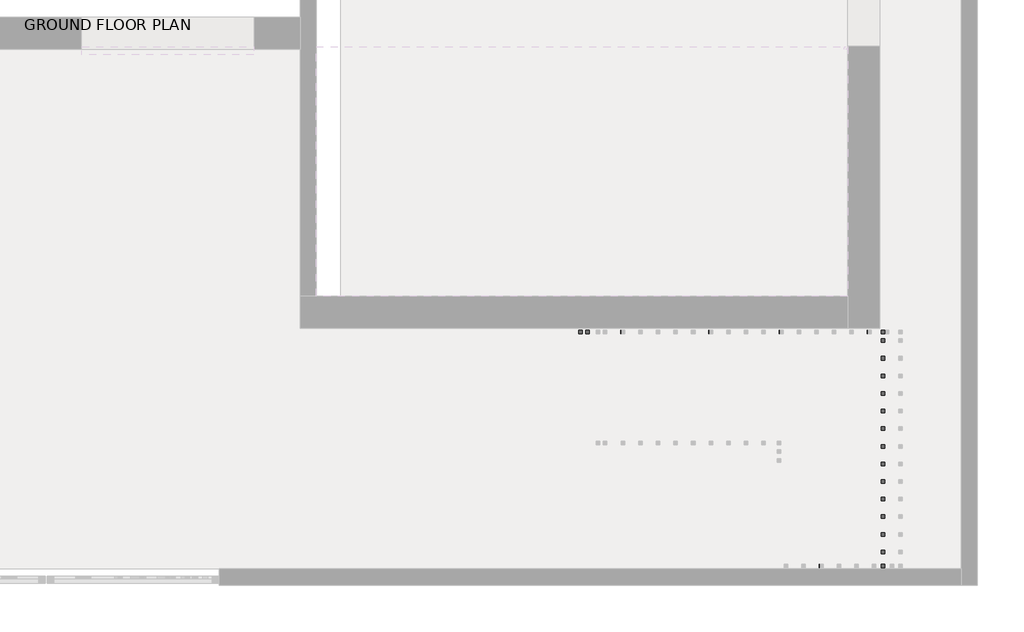
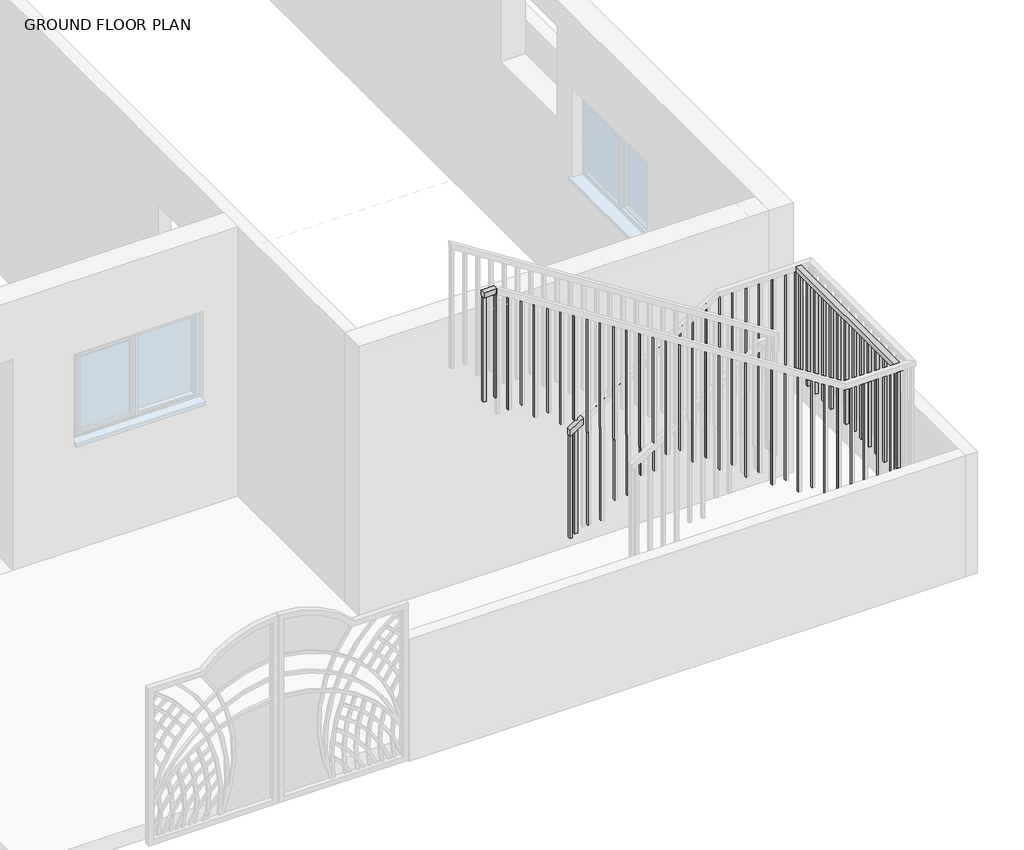
# One storey, part 6 of 23: 2 railings.
"""IFC4 building model written with IfcOpenShell, lengths in millimetres."""

from ifc_helpers import new_model, si_unit, frame, origin, place, context, project, spatial, polyline, outline, extrude, faceted_brep, element, save

model = new_model("IFC4")

# Units and contexts
model_context = context("Model", 3, world=origin())
ifc_project = project(units=[si_unit("LENGTHUNIT", "METRE", prefix="MILLI")], contexts=[model_context])

# Site, building, storey
site = spatial("IfcSite", under=ifc_project)
building = spatial("IfcBuilding", under=site)
storey = spatial("IfcBuildingStorey", under=building, Name="GROUND FLOOR PLAN", Elevation=487.68)

# Railings
placement = place(None, origin())
element("IfcRailing", 1, ObjectType="1100mm", at=placement, inside=storey, context=model_context, shape_type="SolidModel", body=[
    faceted_brep([(-8805.870786, -10220.0521308, 1832.3649576), (-8805.870786, -10220.0521308, 1773.007357), (-8805.870786, -10270.0521308, 1773.007357), (-8805.870786, -10270.0521308, 1832.3649576), (-7409.7306254, -10220.0521308, 2725.6), (-7395.1045513, -10220.0521308, 2675.6), (-7395.1045513, -10270.0521308, 2675.6), (-7409.7306254, -10270.0521308, 2725.6), (-6621.5344696, -10220.0521308, 2725.6), (-6621.5344696, -10220.0521308, 2675.6), (-6671.5344696, -10270.0521308, 2675.6), (-6671.5344696, -10270.0521308, 2725.6), (-6621.5344696, -11933.6860066, 2725.6), (-6621.5344696, -11933.6860066, 2675.6), (-6671.5344696, -11883.6860066, 2675.6), (-6671.5344696, -11883.6860066, 2725.6), (-7155.718398, -11933.6860066, 2725.6), (-7170.3479429, -11933.6860066, 2675.6), (-7170.3479429, -11883.6860066, 2675.6), (-7155.718398, -11883.6860066, 2725.6), (-10457.8773536, -11933.6860066, 4838.88), (-10472.5068984, -11933.6860066, 4788.88), (-10472.5068984, -11883.6860066, 4788.88), (-10457.8773536, -11883.6860066, 4838.88), (-10583.5985666, -11933.6860066, 4838.88), (-10583.5985666, -11883.6860066, 4838.88), (-10583.5985666, -11883.6860066, 4788.88), (-10583.5985666, -11933.6860066, 4788.88)], [[[0, 1, 2, 3]], [[1, 0, 4, 5]], [[2, 1, 5, 6]], [[3, 2, 6, 7]], [[0, 3, 7, 4]], [[5, 4, 8, 9]], [[6, 5, 9, 10]], [[7, 6, 10, 11]], [[4, 7, 11, 8]], [[9, 8, 12, 13]], [[10, 9, 13, 14]], [[11, 10, 14, 15]], [[8, 11, 15, 12]], [[13, 12, 16, 17]], [[14, 13, 17, 18]], [[15, 14, 18, 19]], [[12, 15, 19, 16]], [[17, 16, 20, 21]], [[18, 17, 21, 22]], [[19, 18, 22, 23]], [[16, 19, 23, 20]], [[24, 25, 26, 27]], [[21, 20, 24, 27]], [[22, 21, 27, 26]], [[23, 22, 26, 25]], [[20, 23, 25, 24]]]),
    extrude(outline(polyline([(-10446.5344696, -11921.1860066), (-10471.5344696, -11921.1860066), (-10471.5344696, -11896.1860066), (-10446.5344696, -11896.1860066), (-10446.5344696, -11921.1860066)])), frame((0.0, 0.0, 3738.88), z_axis=(0.0, 0.0, 1.0), x_axis=(1.0, 0.0, 0.0)), (0.0, 0.0, 1.0), 1050.0),
    extrude(outline(polyline([(4692.2622966, -10321.5344696), (4708.2615264, -10346.5344696), (3576.32, -10346.5344696), (3576.32, -10321.5344696), (4692.2622966, -10321.5344696)])), frame((0.0, -11921.1860066, 0.0), z_axis=(0.0, 1.0, 0.0), x_axis=(0.0, 0.0, 1.0)), (0.0, 0.0, 1.0), 25.0),
    extrude(outline(polyline([(4612.2661476, -10196.5344696), (4628.2653774, -10221.5344696), (3576.32, -10221.5344696), (3576.32, -10196.5344696), (4612.2661476, -10196.5344696)])), frame((0.0, -11921.1860066, 0.0), z_axis=(0.0, 1.0, 0.0), x_axis=(0.0, 0.0, 1.0)), (0.0, 0.0, 1.0), 25.0),
    extrude(outline(polyline([(4532.2699985, -10071.5344696), (4548.2692283, -10096.5344696), (3413.76, -10096.5344696), (3413.76, -10071.5344696), (4532.2699985, -10071.5344696)])), frame((0.0, -11921.1860066, 0.0), z_axis=(0.0, 1.0, 0.0), x_axis=(0.0, 0.0, 1.0)), (0.0, 0.0, 1.0), 25.0),
    extrude(outline(polyline([(4452.2738495, -9946.5344696), (4468.2730793, -9971.5344696), (3413.76, -9971.5344696), (3413.76, -9946.5344696), (4452.2738495, -9946.5344696)])), frame((0.0, -11921.1860066, 0.0), z_axis=(0.0, 1.0, 0.0), x_axis=(0.0, 0.0, 1.0)), (0.0, 0.0, 1.0), 25.0),
    extrude(outline(polyline([(4372.2777004, -9821.5344696), (4388.2769302, -9846.5344696), (3251.2, -9846.5344696), (3251.2, -9821.5344696), (4372.2777004, -9821.5344696)])), frame((0.0, -11921.1860066, 0.0), z_axis=(0.0, 1.0, 0.0), x_axis=(0.0, 0.0, 1.0)), (0.0, 0.0, 1.0), 25.0),
    extrude(outline(polyline([(4292.2815514, -9696.5344696), (4308.2807812, -9721.5344696), (3251.2, -9721.5344696), (3251.2, -9696.5344696), (4292.2815514, -9696.5344696)])), frame((0.0, -11921.1860066, 0.0), z_axis=(0.0, 1.0, 0.0), x_axis=(0.0, 0.0, 1.0)), (0.0, 0.0, 1.0), 25.0),
    extrude(outline(polyline([(4212.2854023, -9571.5344696), (4228.2846321, -9596.5344696), (3088.64, -9596.5344696), (3088.64, -9571.5344696), (4212.2854023, -9571.5344696)])), frame((0.0, -11921.1860066, 0.0), z_axis=(0.0, 1.0, 0.0), x_axis=(0.0, 0.0, 1.0)), (0.0, 0.0, 1.0), 25.0),
    extrude(outline(polyline([(4132.2892533, -9446.5344696), (4148.2884831, -9471.5344696), (3088.64, -9471.5344696), (3088.64, -9446.5344696), (4132.2892533, -9446.5344696)])), frame((0.0, -11921.1860066, 0.0), z_axis=(0.0, 1.0, 0.0), x_axis=(0.0, 0.0, 1.0)), (0.0, 0.0, 1.0), 25.0),
    extrude(outline(polyline([(4052.2931042, -9321.5344696), (4068.292334, -9346.5344696), (2926.08, -9346.5344696), (2926.08, -9321.5344696), (4052.2931042, -9321.5344696)])), frame((0.0, -11921.1860066, 0.0), z_axis=(0.0, 1.0, 0.0), x_axis=(0.0, 0.0, 1.0)), (0.0, 0.0, 1.0), 25.0),
    extrude(outline(polyline([(3972.2969552, -9196.5344696), (3988.296185, -9221.5344696), (2926.08, -9221.5344696), (2926.08, -9196.5344696), (3972.2969552, -9196.5344696)])), frame((0.0, -11921.1860066, 0.0), z_axis=(0.0, 1.0, 0.0), x_axis=(0.0, 0.0, 1.0)), (0.0, 0.0, 1.0), 25.0),
    extrude(outline(polyline([(3892.3008061, -9071.5344696), (3908.3000359, -9096.5344696), (2763.52, -9096.5344696), (2763.52, -9071.5344696), (3892.3008061, -9071.5344696)])), frame((0.0, -11921.1860066, 0.0), z_axis=(0.0, 1.0, 0.0), x_axis=(0.0, 0.0, 1.0)), (0.0, 0.0, 1.0), 25.0),
    extrude(outline(polyline([(3812.3046571, -8946.5344696), (3828.3038869, -8971.5344696), (2763.52, -8971.5344696), (2763.52, -8946.5344696), (3812.3046571, -8946.5344696)])), frame((0.0, -11921.1860066, 0.0), z_axis=(0.0, 1.0, 0.0), x_axis=(0.0, 0.0, 1.0)), (0.0, 0.0, 1.0), 25.0),
    extrude(outline(polyline([(3732.308508, -8821.5344696), (3748.3077378, -8846.5344696), (2600.96, -8846.5344696), (2600.96, -8821.5344696), (3732.308508, -8821.5344696)])), frame((0.0, -11921.1860066, 0.0), z_axis=(0.0, 1.0, 0.0), x_axis=(0.0, 0.0, 1.0)), (0.0, 0.0, 1.0), 25.0),
    extrude(outline(polyline([(3652.312359, -8696.5344696), (3668.3115888, -8721.5344696), (2600.96, -8721.5344696), (2600.96, -8696.5344696), (3652.312359, -8696.5344696)])), frame((0.0, -11921.1860066, 0.0), z_axis=(0.0, 1.0, 0.0), x_axis=(0.0, 0.0, 1.0)), (0.0, 0.0, 1.0), 25.0),
    extrude(outline(polyline([(3572.3162099, -8571.5344696), (3588.3154397, -8596.5344696), (2438.4, -8596.5344696), (2438.4, -8571.5344696), (3572.3162099, -8571.5344696)])), frame((0.0, -11921.1860066, 0.0), z_axis=(0.0, 1.0, 0.0), x_axis=(0.0, 0.0, 1.0)), (0.0, 0.0, 1.0), 25.0),
    extrude(outline(polyline([(3492.3200609, -8446.5344696), (3508.3192907, -8471.5344696), (2438.4, -8471.5344696), (2438.4, -8446.5344696), (3492.3200609, -8446.5344696)])), frame((0.0, -11921.1860066, 0.0), z_axis=(0.0, 1.0, 0.0), x_axis=(0.0, 0.0, 1.0)), (0.0, 0.0, 1.0), 25.0),
    extrude(outline(polyline([(3412.3239118, -8321.5344696), (3428.3231416, -8346.5344696), (2275.84, -8346.5344696), (2275.84, -8321.5344696), (3412.3239118, -8321.5344696)])), frame((0.0, -11921.1860066, 0.0), z_axis=(0.0, 1.0, 0.0), x_axis=(0.0, 0.0, 1.0)), (0.0, 0.0, 1.0), 25.0),
    extrude(outline(polyline([(3332.3277628, -8196.5344696), (3348.3269926, -8221.5344696), (2275.84, -8221.5344696), (2275.84, -8196.5344696), (3332.3277628, -8196.5344696)])), frame((0.0, -11921.1860066, 0.0), z_axis=(0.0, 1.0, 0.0), x_axis=(0.0, 0.0, 1.0)), (0.0, 0.0, 1.0), 25.0),
    extrude(outline(polyline([(3252.3316137, -8071.5344696), (3268.3308435, -8096.5344696), (2113.28, -8096.5344696), (2113.28, -8071.5344696), (3252.3316137, -8071.5344696)])), frame((0.0, -11921.1860066, 0.0), z_axis=(0.0, 1.0, 0.0), x_axis=(0.0, 0.0, 1.0)), (0.0, 0.0, 1.0), 25.0),
    extrude(outline(polyline([(3172.3354647, -7946.5344696), (3188.3346945, -7971.5344696), (2113.28, -7971.5344696), (2113.28, -7946.5344696), (3172.3354647, -7946.5344696)])), frame((0.0, -11921.1860066, 0.0), z_axis=(0.0, 1.0, 0.0), x_axis=(0.0, 0.0, 1.0)), (0.0, 0.0, 1.0), 25.0),
    extrude(outline(polyline([(3092.4129874, -7821.5344696), (3108.4077111, -7846.5344696), (1950.72, -7846.5344696), (1950.72, -7821.5344696), (3092.4129874, -7821.5344696)])), frame((0.0, -11921.1860066, 0.0), z_axis=(0.0, 1.0, 0.0), x_axis=(0.0, 0.0, 1.0)), (0.0, 0.0, 1.0), 25.0),
    extrude(outline(polyline([(3012.4393691, -7696.5344696), (3028.4340928, -7721.5344696), (1950.72, -7721.5344696), (1950.72, -7696.5344696), (3012.4393691, -7696.5344696)])), frame((0.0, -11921.1860066, 0.0), z_axis=(0.0, 1.0, 0.0), x_axis=(0.0, 0.0, 1.0)), (0.0, 0.0, 1.0), 25.0),
    extrude(outline(polyline([(2932.4657508, -7571.5344696), (2948.4604745, -7596.5344696), (1788.16, -7596.5344696), (1788.16, -7571.5344696), (2932.4657508, -7571.5344696)])), frame((0.0, -11921.1860066, 0.0), z_axis=(0.0, 1.0, 0.0), x_axis=(0.0, 0.0, 1.0)), (0.0, 0.0, 1.0), 25.0),
    extrude(outline(polyline([(2852.4921325, -7446.5344696), (2868.4868562, -7471.5344696), (1788.16, -7471.5344696), (1788.16, -7446.5344696), (2852.4921325, -7446.5344696)])), frame((0.0, -11921.1860066, 0.0), z_axis=(0.0, 1.0, 0.0), x_axis=(0.0, 0.0, 1.0)), (0.0, 0.0, 1.0), 25.0),
    extrude(outline(polyline([(2772.3547194, -7321.5344696), (2788.3539492, -7346.5344696), (1625.6, -7346.5344696), (1625.6, -7321.5344696), (2772.3547194, -7321.5344696)])), frame((0.0, -11921.1860066, 0.0), z_axis=(0.0, 1.0, 0.0), x_axis=(0.0, 0.0, 1.0)), (0.0, 0.0, 1.0), 25.0),
    extrude(outline(polyline([(2692.3585703, -7196.5344696), (2708.3578001, -7221.5344696), (1625.6, -7221.5344696), (1625.6, -7196.5344696), (2692.3585703, -7196.5344696)])), frame((0.0, -11921.1860066, 0.0), z_axis=(0.0, 1.0, 0.0), x_axis=(0.0, 0.0, 1.0)), (0.0, 0.0, 1.0), 25.0),
    extrude(outline(polyline([(-7071.5344696, -11921.1860066), (-7096.5344696, -11921.1860066), (-7096.5344696, -11896.1860066), (-7071.5344696, -11896.1860066), (-7071.5344696, -11921.1860066)])), frame((0.0, 0.0, 1625.6), z_axis=(0.0, 0.0, 1.0), x_axis=(1.0, 0.0, 0.0)), (0.0, 0.0, 1.0), 1050.0),
    extrude(outline(polyline([(-6946.5344696, -11921.1860066), (-6971.5344696, -11921.1860066), (-6971.5344696, -11896.1860066), (-6946.5344696, -11896.1860066), (-6946.5344696, -11921.1860066)])), frame((0.0, 0.0, 1625.6), z_axis=(0.0, 0.0, 1.0), x_axis=(1.0, 0.0, 0.0)), (0.0, 0.0, 1.0), 1050.0),
    extrude(outline(polyline([(-6821.5344696, -11921.1860066), (-6846.5344696, -11921.1860066), (-6846.5344696, -11896.1860066), (-6821.5344696, -11896.1860066), (-6821.5344696, -11921.1860066)])), frame((0.0, 0.0, 1625.6), z_axis=(0.0, 0.0, 1.0), x_axis=(1.0, 0.0, 0.0)), (0.0, 0.0, 1.0), 1050.0),
    extrude(outline(polyline([(-6696.5344696, -11921.1860066), (-6721.5344696, -11921.1860066), (-6721.5344696, -11896.1860066), (-6696.5344696, -11896.1860066), (-6696.5344696, -11921.1860066)])), frame((0.0, 0.0, 1625.6), z_axis=(0.0, 0.0, 1.0), x_axis=(1.0, 0.0, 0.0)), (0.0, 0.0, 1.0), 1050.0),
    extrude(outline(polyline([(-6634.0344696, -11795.0521308), (-6634.0344696, -11820.0521308), (-6659.0344696, -11820.0521308), (-6659.0344696, -11795.0521308), (-6634.0344696, -11795.0521308)])), frame((0.0, 0.0, 1625.6), z_axis=(0.0, 0.0, 1.0), x_axis=(1.0, 0.0, 0.0)), (0.0, 0.0, 1.0), 1050.0),
    extrude(outline(polyline([(-6634.0344696, -11670.0521308), (-6634.0344696, -11695.0521308), (-6659.0344696, -11695.0521308), (-6659.0344696, -11670.0521308), (-6634.0344696, -11670.0521308)])), frame((0.0, 0.0, 1625.6), z_axis=(0.0, 0.0, 1.0), x_axis=(1.0, 0.0, 0.0)), (0.0, 0.0, 1.0), 1050.0),
    extrude(outline(polyline([(-6634.0344696, -11545.0521308), (-6634.0344696, -11570.0521308), (-6659.0344696, -11570.0521308), (-6659.0344696, -11545.0521308), (-6634.0344696, -11545.0521308)])), frame((0.0, 0.0, 1625.6), z_axis=(0.0, 0.0, 1.0), x_axis=(1.0, 0.0, 0.0)), (0.0, 0.0, 1.0), 1050.0),
    extrude(outline(polyline([(-6634.0344696, -11420.0521308), (-6634.0344696, -11445.0521308), (-6659.0344696, -11445.0521308), (-6659.0344696, -11420.0521308), (-6634.0344696, -11420.0521308)])), frame((0.0, 0.0, 1625.6), z_axis=(0.0, 0.0, 1.0), x_axis=(1.0, 0.0, 0.0)), (0.0, 0.0, 1.0), 1050.0),
    extrude(outline(polyline([(-6634.0344696, -11295.0521308), (-6634.0344696, -11320.0521308), (-6659.0344696, -11320.0521308), (-6659.0344696, -11295.0521308), (-6634.0344696, -11295.0521308)])), frame((0.0, 0.0, 1625.6), z_axis=(0.0, 0.0, 1.0), x_axis=(1.0, 0.0, 0.0)), (0.0, 0.0, 1.0), 1050.0),
    extrude(outline(polyline([(-6634.0344696, -11170.0521308), (-6634.0344696, -11195.0521308), (-6659.0344696, -11195.0521308), (-6659.0344696, -11170.0521308), (-6634.0344696, -11170.0521308)])), frame((0.0, 0.0, 1625.6), z_axis=(0.0, 0.0, 1.0), x_axis=(1.0, 0.0, 0.0)), (0.0, 0.0, 1.0), 1050.0),
    extrude(outline(polyline([(-6634.0344696, -11045.0521308), (-6634.0344696, -11070.0521308), (-6659.0344696, -11070.0521308), (-6659.0344696, -11045.0521308), (-6634.0344696, -11045.0521308)])), frame((0.0, 0.0, 1625.6), z_axis=(0.0, 0.0, 1.0), x_axis=(1.0, 0.0, 0.0)), (0.0, 0.0, 1.0), 1050.0),
    extrude(outline(polyline([(-6634.0344696, -10920.0521308), (-6634.0344696, -10945.0521308), (-6659.0344696, -10945.0521308), (-6659.0344696, -10920.0521308), (-6634.0344696, -10920.0521308)])), frame((0.0, 0.0, 1625.6), z_axis=(0.0, 0.0, 1.0), x_axis=(1.0, 0.0, 0.0)), (0.0, 0.0, 1.0), 1050.0),
    extrude(outline(polyline([(-6634.0344696, -10795.0521308), (-6634.0344696, -10820.0521308), (-6659.0344696, -10820.0521308), (-6659.0344696, -10795.0521308), (-6634.0344696, -10795.0521308)])), frame((0.0, 0.0, 1625.6), z_axis=(0.0, 0.0, 1.0), x_axis=(1.0, 0.0, 0.0)), (0.0, 0.0, 1.0), 1050.0),
    extrude(outline(polyline([(-6634.0344696, -10670.0521308), (-6634.0344696, -10695.0521308), (-6659.0344696, -10695.0521308), (-6659.0344696, -10670.0521308), (-6634.0344696, -10670.0521308)])), frame((0.0, 0.0, 1625.6), z_axis=(0.0, 0.0, 1.0), x_axis=(1.0, 0.0, 0.0)), (0.0, 0.0, 1.0), 1050.0),
    extrude(outline(polyline([(-6634.0344696, -10545.0521308), (-6634.0344696, -10570.0521308), (-6659.0344696, -10570.0521308), (-6659.0344696, -10545.0521308), (-6634.0344696, -10545.0521308)])), frame((0.0, 0.0, 1625.6), z_axis=(0.0, 0.0, 1.0), x_axis=(1.0, 0.0, 0.0)), (0.0, 0.0, 1.0), 1050.0),
    extrude(outline(polyline([(-6634.0344696, -10420.0521308), (-6634.0344696, -10445.0521308), (-6659.0344696, -10445.0521308), (-6659.0344696, -10420.0521308), (-6634.0344696, -10420.0521308)])), frame((0.0, 0.0, 1625.6), z_axis=(0.0, 0.0, 1.0), x_axis=(1.0, 0.0, 0.0)), (0.0, 0.0, 1.0), 1050.0),
    extrude(outline(polyline([(-6634.0344696, -10295.0521308), (-6634.0344696, -10320.0521308), (-6659.0344696, -10320.0521308), (-6659.0344696, -10295.0521308), (-6634.0344696, -10295.0521308)])), frame((0.0, 0.0, 1625.6), z_axis=(0.0, 0.0, 1.0), x_axis=(1.0, 0.0, 0.0)), (0.0, 0.0, 1.0), 1050.0),
    extrude(outline(polyline([(-6755.870786, -10232.5521308), (-6730.870786, -10232.5521308), (-6730.870786, -10257.5521308), (-6755.870786, -10257.5521308), (-6755.870786, -10232.5521308)])), frame((0.0, 0.0, 1625.6), z_axis=(0.0, 0.0, 1.0), x_axis=(1.0, 0.0, 0.0)), (0.0, 0.0, 1.0), 1050.0),
    extrude(outline(polyline([(-6880.870786, -10232.5521308), (-6855.870786, -10232.5521308), (-6855.870786, -10257.5521308), (-6880.870786, -10257.5521308), (-6880.870786, -10232.5521308)])), frame((0.0, 0.0, 1625.6), z_axis=(0.0, 0.0, 1.0), x_axis=(1.0, 0.0, 0.0)), (0.0, 0.0, 1.0), 1050.0),
    extrude(outline(polyline([(-7005.870786, -10232.5521308), (-6980.870786, -10232.5521308), (-6980.870786, -10257.5521308), (-7005.870786, -10257.5521308), (-7005.870786, -10232.5521308)])), frame((0.0, 0.0, 1625.6), z_axis=(0.0, 0.0, 1.0), x_axis=(1.0, 0.0, 0.0)), (0.0, 0.0, 1.0), 1050.0),
    extrude(outline(polyline([(-7130.870786, -10232.5521308), (-7105.870786, -10232.5521308), (-7105.870786, -10257.5521308), (-7130.870786, -10257.5521308), (-7130.870786, -10232.5521308)])), frame((0.0, 0.0, 1625.6), z_axis=(0.0, 0.0, 1.0), x_axis=(1.0, 0.0, 0.0)), (0.0, 0.0, 1.0), 1050.0),
    extrude(outline(polyline([(-7255.870786, -10232.5521308), (-7230.870786, -10232.5521308), (-7230.870786, -10257.5521308), (-7255.870786, -10257.5521308), (-7255.870786, -10232.5521308)])), frame((0.0, 0.0, 1625.6), z_axis=(0.0, 0.0, 1.0), x_axis=(1.0, 0.0, 0.0)), (0.0, 0.0, 1.0), 1050.0),
    extrude(outline(polyline([(-7380.870786, -10232.5521308), (-7355.870786, -10232.5521308), (-7355.870786, -10257.5521308), (-7380.870786, -10257.5521308), (-7380.870786, -10232.5521308)])), frame((0.0, 0.0, 1625.6), z_axis=(0.0, 0.0, 1.0), x_axis=(1.0, 0.0, 0.0)), (0.0, 0.0, 1.0), 1050.0),
    extrude(outline(polyline([(1463.04, -7505.870786), (1463.04, -7480.870786), (2620.7277111, -7480.870786), (2604.7329874, -7505.870786), (1463.04, -7505.870786)])), frame((0.0, -10257.5521308, 0.0), z_axis=(0.0, 1.0, 0.0), x_axis=(0.0, 0.0, 1.0)), (0.0, 0.0, 1.0), 25.0),
    extrude(outline(polyline([(1463.04, -7630.870786), (1463.04, -7605.870786), (2540.7540928, -7605.870786), (2524.7593691, -7630.870786), (1463.04, -7630.870786)])), frame((0.0, -10257.5521308, 0.0), z_axis=(0.0, 1.0, 0.0), x_axis=(0.0, 0.0, 1.0)), (0.0, 0.0, 1.0), 25.0),
    extrude(outline(polyline([(1300.48, -7755.870786), (1300.48, -7730.870786), (2460.7804745, -7730.870786), (2444.7857508, -7755.870786), (1300.48, -7755.870786)])), frame((0.0, -10257.5521308, 0.0), z_axis=(0.0, 1.0, 0.0), x_axis=(0.0, 0.0, 1.0)), (0.0, 0.0, 1.0), 25.0),
    extrude(outline(polyline([(1300.48, -7880.870786), (1300.48, -7855.870786), (2380.8068562, -7855.870786), (2364.8121325, -7880.870786), (1300.48, -7880.870786)])), frame((0.0, -10257.5521308, 0.0), z_axis=(0.0, 1.0, 0.0), x_axis=(0.0, 0.0, 1.0)), (0.0, 0.0, 1.0), 25.0),
    extrude(outline(polyline([(1137.92, -8005.870786), (1137.92, -7980.870786), (2300.8332379, -7980.870786), (2284.8385142, -8005.870786), (1137.92, -8005.870786)])), frame((0.0, -10257.5521308, 0.0), z_axis=(0.0, 1.0, 0.0), x_axis=(0.0, 0.0, 1.0)), (0.0, 0.0, 1.0), 25.0),
    extrude(outline(polyline([(1137.92, -8130.870786), (1137.92, -8105.870786), (2220.8596196, -8105.870786), (2204.8648959, -8130.870786), (1137.92, -8130.870786)])), frame((0.0, -10257.5521308, 0.0), z_axis=(0.0, 1.0, 0.0), x_axis=(0.0, 0.0, 1.0)), (0.0, 0.0, 1.0), 25.0),
    extrude(outline(polyline([(975.36, -8255.870786), (975.36, -8230.870786), (2140.8860012, -8230.870786), (2124.8912776, -8255.870786), (975.36, -8255.870786)])), frame((0.0, -10257.5521308, 0.0), z_axis=(0.0, 1.0, 0.0), x_axis=(0.0, 0.0, 1.0)), (0.0, 0.0, 1.0), 25.0),
    extrude(outline(polyline([(975.36, -8380.870786), (975.36, -8355.870786), (2060.9123829, -8355.870786), (2044.9176593, -8380.870786), (975.36, -8380.870786)])), frame((0.0, -10257.5521308, 0.0), z_axis=(0.0, 1.0, 0.0), x_axis=(0.0, 0.0, 1.0)), (0.0, 0.0, 1.0), 25.0),
    extrude(outline(polyline([(812.8, -8505.870786), (812.8, -8480.870786), (1980.9387646, -8480.870786), (1964.944041, -8505.870786), (812.8, -8505.870786)])), frame((0.0, -10257.5521308, 0.0), z_axis=(0.0, 1.0, 0.0), x_axis=(0.0, 0.0, 1.0)), (0.0, 0.0, 1.0), 25.0),
    extrude(outline(polyline([(812.8, -8630.870786), (812.8, -8605.870786), (1900.9651463, -8605.870786), (1884.9704227, -8630.870786), (812.8, -8630.870786)])), frame((0.0, -10257.5521308, 0.0), z_axis=(0.0, 1.0, 0.0), x_axis=(0.0, 0.0, 1.0)), (0.0, 0.0, 1.0), 25.0),
    extrude(outline(polyline([(772.3517667, -8755.870786), (772.3517667, -8730.870786), (1820.991528, -8730.870786), (1804.9968044, -8755.870786), (772.3517667, -8755.870786)])), frame((0.0, -10257.5521308, 0.0), z_axis=(0.0, 1.0, 0.0), x_axis=(0.0, 0.0, 1.0)), (0.0, 0.0, 1.0), 25.0),
    extrude(outline(polyline([(-6634.0344696, -11896.1860066), (-6634.0344696, -11921.1860066), (-6659.0344696, -11921.1860066), (-6659.0344696, -11896.1860066), (-6634.0344696, -11896.1860066)])), frame((0.0, 0.0, 1625.6), z_axis=(0.0, 0.0, 1.0), x_axis=(1.0, 0.0, 0.0)), (0.0, 0.0, 1.0), 1050.0),
    extrude(outline(polyline([(-6659.0344696, -10232.5521308), (-6634.0344696, -10232.5521308), (-6634.0344696, -10257.5521308), (-6659.0344696, -10257.5521308), (-6659.0344696, -10232.5521308)])), frame((0.0, 0.0, 1625.6), z_axis=(0.0, 0.0, 1.0), x_axis=(1.0, 0.0, 0.0)), (0.0, 0.0, 1.0), 1050.0),
    extrude(outline(polyline([(-10558.5985666, -11921.1860066), (-10583.5985666, -11921.1860066), (-10583.5985666, -11896.1860066), (-10558.5985666, -11896.1860066), (-10558.5985666, -11921.1860066)])), frame((0.0, 0.0, 3738.88), z_axis=(0.0, 0.0, 1.0), x_axis=(1.0, 0.0, 0.0)), (0.0, 0.0, 1.0), 1050.0),
    extrude(outline(polyline([(740.3623194, -8805.870786), (740.3623194, -8780.870786), (1789.0020807, -8780.870786), (1773.007357, -8805.870786), (740.3623194, -8805.870786)])), frame((0.0, -10257.5521308, 0.0), z_axis=(0.0, 1.0, 0.0), x_axis=(0.0, 0.0, 1.0)), (0.0, 0.0, 1.0), 25.0),
])
element("IfcRailing", 2, ObjectType="1100mm", at=placement, inside=storey, context=model_context, shape_type="SolidModel", body=[
    faceted_brep([(-8805.870786, -10220.0521308, 1832.3649576), (-8805.870786, -10220.0521308, 1773.007357), (-8805.870786, -10270.0521308, 1773.007357), (-8805.870786, -10270.0521308, 1832.3649576), (-7409.7306254, -10220.0521308, 2725.6), (-7395.1045513, -10220.0521308, 2675.6), (-7395.1045513, -10270.0521308, 2675.6), (-7409.7306254, -10270.0521308, 2725.6), (-6621.5344696, -10220.0521308, 2725.6), (-6621.5344696, -10220.0521308, 2675.6), (-6671.5344696, -10270.0521308, 2675.6), (-6671.5344696, -10270.0521308, 2725.6), (-6621.5344696, -11933.6860066, 2725.6), (-6621.5344696, -11933.6860066, 2675.6), (-6671.5344696, -11883.6860066, 2675.6), (-6671.5344696, -11883.6860066, 2725.6), (-7155.718398, -11933.6860066, 2725.6), (-7170.3479429, -11933.6860066, 2675.6), (-7170.3479429, -11883.6860066, 2675.6), (-7155.718398, -11883.6860066, 2725.6), (-10457.8773536, -11933.6860066, 4838.88), (-10472.5068984, -11933.6860066, 4788.88), (-10472.5068984, -11883.6860066, 4788.88), (-10457.8773536, -11883.6860066, 4838.88), (-10583.5985666, -11933.6860066, 4838.88), (-10583.5985666, -11883.6860066, 4838.88), (-10583.5985666, -11883.6860066, 4788.88), (-10583.5985666, -11933.6860066, 4788.88)], [[[0, 1, 2, 3]], [[1, 0, 4, 5]], [[2, 1, 5, 6]], [[3, 2, 6, 7]], [[0, 3, 7, 4]], [[5, 4, 8, 9]], [[6, 5, 9, 10]], [[7, 6, 10, 11]], [[4, 7, 11, 8]], [[9, 8, 12, 13]], [[10, 9, 13, 14]], [[11, 10, 14, 15]], [[8, 11, 15, 12]], [[13, 12, 16, 17]], [[14, 13, 17, 18]], [[15, 14, 18, 19]], [[12, 15, 19, 16]], [[17, 16, 20, 21]], [[18, 17, 21, 22]], [[19, 18, 22, 23]], [[16, 19, 23, 20]], [[24, 25, 26, 27]], [[21, 20, 24, 27]], [[22, 21, 27, 26]], [[23, 22, 26, 25]], [[20, 23, 25, 24]]]),
    extrude(outline(polyline([(-10446.5344696, -11921.1860066), (-10471.5344696, -11921.1860066), (-10471.5344696, -11896.1860066), (-10446.5344696, -11896.1860066), (-10446.5344696, -11921.1860066)])), frame((0.0, 0.0, 3738.88), z_axis=(0.0, 0.0, 1.0), x_axis=(1.0, 0.0, 0.0)), (0.0, 0.0, 1.0), 1050.0),
    extrude(outline(polyline([(4692.2622966, -10321.5344696), (4708.2615264, -10346.5344696), (3576.32, -10346.5344696), (3576.32, -10321.5344696), (4692.2622966, -10321.5344696)])), frame((0.0, -11921.1860066, 0.0), z_axis=(0.0, 1.0, 0.0), x_axis=(0.0, 0.0, 1.0)), (0.0, 0.0, 1.0), 25.0),
    extrude(outline(polyline([(4612.2661476, -10196.5344696), (4628.2653774, -10221.5344696), (3576.32, -10221.5344696), (3576.32, -10196.5344696), (4612.2661476, -10196.5344696)])), frame((0.0, -11921.1860066, 0.0), z_axis=(0.0, 1.0, 0.0), x_axis=(0.0, 0.0, 1.0)), (0.0, 0.0, 1.0), 25.0),
    extrude(outline(polyline([(4532.2699985, -10071.5344696), (4548.2692283, -10096.5344696), (3413.76, -10096.5344696), (3413.76, -10071.5344696), (4532.2699985, -10071.5344696)])), frame((0.0, -11921.1860066, 0.0), z_axis=(0.0, 1.0, 0.0), x_axis=(0.0, 0.0, 1.0)), (0.0, 0.0, 1.0), 25.0),
    extrude(outline(polyline([(4452.2738495, -9946.5344696), (4468.2730793, -9971.5344696), (3413.76, -9971.5344696), (3413.76, -9946.5344696), (4452.2738495, -9946.5344696)])), frame((0.0, -11921.1860066, 0.0), z_axis=(0.0, 1.0, 0.0), x_axis=(0.0, 0.0, 1.0)), (0.0, 0.0, 1.0), 25.0),
    extrude(outline(polyline([(4372.2777004, -9821.5344696), (4388.2769302, -9846.5344696), (3251.2, -9846.5344696), (3251.2, -9821.5344696), (4372.2777004, -9821.5344696)])), frame((0.0, -11921.1860066, 0.0), z_axis=(0.0, 1.0, 0.0), x_axis=(0.0, 0.0, 1.0)), (0.0, 0.0, 1.0), 25.0),
    extrude(outline(polyline([(4292.2815514, -9696.5344696), (4308.2807812, -9721.5344696), (3251.2, -9721.5344696), (3251.2, -9696.5344696), (4292.2815514, -9696.5344696)])), frame((0.0, -11921.1860066, 0.0), z_axis=(0.0, 1.0, 0.0), x_axis=(0.0, 0.0, 1.0)), (0.0, 0.0, 1.0), 25.0),
    extrude(outline(polyline([(4212.2854023, -9571.5344696), (4228.2846321, -9596.5344696), (3088.64, -9596.5344696), (3088.64, -9571.5344696), (4212.2854023, -9571.5344696)])), frame((0.0, -11921.1860066, 0.0), z_axis=(0.0, 1.0, 0.0), x_axis=(0.0, 0.0, 1.0)), (0.0, 0.0, 1.0), 25.0),
    extrude(outline(polyline([(4132.2892533, -9446.5344696), (4148.2884831, -9471.5344696), (3088.64, -9471.5344696), (3088.64, -9446.5344696), (4132.2892533, -9446.5344696)])), frame((0.0, -11921.1860066, 0.0), z_axis=(0.0, 1.0, 0.0), x_axis=(0.0, 0.0, 1.0)), (0.0, 0.0, 1.0), 25.0),
    extrude(outline(polyline([(4052.2931042, -9321.5344696), (4068.292334, -9346.5344696), (2926.08, -9346.5344696), (2926.08, -9321.5344696), (4052.2931042, -9321.5344696)])), frame((0.0, -11921.1860066, 0.0), z_axis=(0.0, 1.0, 0.0), x_axis=(0.0, 0.0, 1.0)), (0.0, 0.0, 1.0), 25.0),
    extrude(outline(polyline([(3972.2969552, -9196.5344696), (3988.296185, -9221.5344696), (2926.08, -9221.5344696), (2926.08, -9196.5344696), (3972.2969552, -9196.5344696)])), frame((0.0, -11921.1860066, 0.0), z_axis=(0.0, 1.0, 0.0), x_axis=(0.0, 0.0, 1.0)), (0.0, 0.0, 1.0), 25.0),
    extrude(outline(polyline([(3892.3008061, -9071.5344696), (3908.3000359, -9096.5344696), (2763.52, -9096.5344696), (2763.52, -9071.5344696), (3892.3008061, -9071.5344696)])), frame((0.0, -11921.1860066, 0.0), z_axis=(0.0, 1.0, 0.0), x_axis=(0.0, 0.0, 1.0)), (0.0, 0.0, 1.0), 25.0),
    extrude(outline(polyline([(3812.3046571, -8946.5344696), (3828.3038869, -8971.5344696), (2763.52, -8971.5344696), (2763.52, -8946.5344696), (3812.3046571, -8946.5344696)])), frame((0.0, -11921.1860066, 0.0), z_axis=(0.0, 1.0, 0.0), x_axis=(0.0, 0.0, 1.0)), (0.0, 0.0, 1.0), 25.0),
    extrude(outline(polyline([(3732.308508, -8821.5344696), (3748.3077378, -8846.5344696), (2600.96, -8846.5344696), (2600.96, -8821.5344696), (3732.308508, -8821.5344696)])), frame((0.0, -11921.1860066, 0.0), z_axis=(0.0, 1.0, 0.0), x_axis=(0.0, 0.0, 1.0)), (0.0, 0.0, 1.0), 25.0),
    extrude(outline(polyline([(3652.312359, -8696.5344696), (3668.3115888, -8721.5344696), (2600.96, -8721.5344696), (2600.96, -8696.5344696), (3652.312359, -8696.5344696)])), frame((0.0, -11921.1860066, 0.0), z_axis=(0.0, 1.0, 0.0), x_axis=(0.0, 0.0, 1.0)), (0.0, 0.0, 1.0), 25.0),
    extrude(outline(polyline([(3572.3162099, -8571.5344696), (3588.3154397, -8596.5344696), (2438.4, -8596.5344696), (2438.4, -8571.5344696), (3572.3162099, -8571.5344696)])), frame((0.0, -11921.1860066, 0.0), z_axis=(0.0, 1.0, 0.0), x_axis=(0.0, 0.0, 1.0)), (0.0, 0.0, 1.0), 25.0),
    extrude(outline(polyline([(3492.3200609, -8446.5344696), (3508.3192907, -8471.5344696), (2438.4, -8471.5344696), (2438.4, -8446.5344696), (3492.3200609, -8446.5344696)])), frame((0.0, -11921.1860066, 0.0), z_axis=(0.0, 1.0, 0.0), x_axis=(0.0, 0.0, 1.0)), (0.0, 0.0, 1.0), 25.0),
    extrude(outline(polyline([(3412.3239118, -8321.5344696), (3428.3231416, -8346.5344696), (2275.84, -8346.5344696), (2275.84, -8321.5344696), (3412.3239118, -8321.5344696)])), frame((0.0, -11921.1860066, 0.0), z_axis=(0.0, 1.0, 0.0), x_axis=(0.0, 0.0, 1.0)), (0.0, 0.0, 1.0), 25.0),
    extrude(outline(polyline([(3332.3277628, -8196.5344696), (3348.3269926, -8221.5344696), (2275.84, -8221.5344696), (2275.84, -8196.5344696), (3332.3277628, -8196.5344696)])), frame((0.0, -11921.1860066, 0.0), z_axis=(0.0, 1.0, 0.0), x_axis=(0.0, 0.0, 1.0)), (0.0, 0.0, 1.0), 25.0),
    extrude(outline(polyline([(3252.3316137, -8071.5344696), (3268.3308435, -8096.5344696), (2113.28, -8096.5344696), (2113.28, -8071.5344696), (3252.3316137, -8071.5344696)])), frame((0.0, -11921.1860066, 0.0), z_axis=(0.0, 1.0, 0.0), x_axis=(0.0, 0.0, 1.0)), (0.0, 0.0, 1.0), 25.0),
    extrude(outline(polyline([(3172.3354647, -7946.5344696), (3188.3346945, -7971.5344696), (2113.28, -7971.5344696), (2113.28, -7946.5344696), (3172.3354647, -7946.5344696)])), frame((0.0, -11921.1860066, 0.0), z_axis=(0.0, 1.0, 0.0), x_axis=(0.0, 0.0, 1.0)), (0.0, 0.0, 1.0), 25.0),
    extrude(outline(polyline([(3092.4129874, -7821.5344696), (3108.4077111, -7846.5344696), (1950.72, -7846.5344696), (1950.72, -7821.5344696), (3092.4129874, -7821.5344696)])), frame((0.0, -11921.1860066, 0.0), z_axis=(0.0, 1.0, 0.0), x_axis=(0.0, 0.0, 1.0)), (0.0, 0.0, 1.0), 25.0),
    extrude(outline(polyline([(3012.4393691, -7696.5344696), (3028.4340928, -7721.5344696), (1950.72, -7721.5344696), (1950.72, -7696.5344696), (3012.4393691, -7696.5344696)])), frame((0.0, -11921.1860066, 0.0), z_axis=(0.0, 1.0, 0.0), x_axis=(0.0, 0.0, 1.0)), (0.0, 0.0, 1.0), 25.0),
    extrude(outline(polyline([(2932.4657508, -7571.5344696), (2948.4604745, -7596.5344696), (1788.16, -7596.5344696), (1788.16, -7571.5344696), (2932.4657508, -7571.5344696)])), frame((0.0, -11921.1860066, 0.0), z_axis=(0.0, 1.0, 0.0), x_axis=(0.0, 0.0, 1.0)), (0.0, 0.0, 1.0), 25.0),
    extrude(outline(polyline([(2852.4921325, -7446.5344696), (2868.4868562, -7471.5344696), (1788.16, -7471.5344696), (1788.16, -7446.5344696), (2852.4921325, -7446.5344696)])), frame((0.0, -11921.1860066, 0.0), z_axis=(0.0, 1.0, 0.0), x_axis=(0.0, 0.0, 1.0)), (0.0, 0.0, 1.0), 25.0),
    extrude(outline(polyline([(2772.3547194, -7321.5344696), (2788.3539492, -7346.5344696), (1625.6, -7346.5344696), (1625.6, -7321.5344696), (2772.3547194, -7321.5344696)])), frame((0.0, -11921.1860066, 0.0), z_axis=(0.0, 1.0, 0.0), x_axis=(0.0, 0.0, 1.0)), (0.0, 0.0, 1.0), 25.0),
    extrude(outline(polyline([(2692.3585703, -7196.5344696), (2708.3578001, -7221.5344696), (1625.6, -7221.5344696), (1625.6, -7196.5344696), (2692.3585703, -7196.5344696)])), frame((0.0, -11921.1860066, 0.0), z_axis=(0.0, 1.0, 0.0), x_axis=(0.0, 0.0, 1.0)), (0.0, 0.0, 1.0), 25.0),
    extrude(outline(polyline([(-7071.5344696, -11921.1860066), (-7096.5344696, -11921.1860066), (-7096.5344696, -11896.1860066), (-7071.5344696, -11896.1860066), (-7071.5344696, -11921.1860066)])), frame((0.0, 0.0, 1625.6), z_axis=(0.0, 0.0, 1.0), x_axis=(1.0, 0.0, 0.0)), (0.0, 0.0, 1.0), 1050.0),
    extrude(outline(polyline([(-6946.5344696, -11921.1860066), (-6971.5344696, -11921.1860066), (-6971.5344696, -11896.1860066), (-6946.5344696, -11896.1860066), (-6946.5344696, -11921.1860066)])), frame((0.0, 0.0, 1625.6), z_axis=(0.0, 0.0, 1.0), x_axis=(1.0, 0.0, 0.0)), (0.0, 0.0, 1.0), 1050.0),
    extrude(outline(polyline([(-6821.5344696, -11921.1860066), (-6846.5344696, -11921.1860066), (-6846.5344696, -11896.1860066), (-6821.5344696, -11896.1860066), (-6821.5344696, -11921.1860066)])), frame((0.0, 0.0, 1625.6), z_axis=(0.0, 0.0, 1.0), x_axis=(1.0, 0.0, 0.0)), (0.0, 0.0, 1.0), 1050.0),
    extrude(outline(polyline([(-6696.5344696, -11921.1860066), (-6721.5344696, -11921.1860066), (-6721.5344696, -11896.1860066), (-6696.5344696, -11896.1860066), (-6696.5344696, -11921.1860066)])), frame((0.0, 0.0, 1625.6), z_axis=(0.0, 0.0, 1.0), x_axis=(1.0, 0.0, 0.0)), (0.0, 0.0, 1.0), 1050.0),
    extrude(outline(polyline([(-6634.0344696, -11795.0521308), (-6634.0344696, -11820.0521308), (-6659.0344696, -11820.0521308), (-6659.0344696, -11795.0521308), (-6634.0344696, -11795.0521308)])), frame((0.0, 0.0, 1625.6), z_axis=(0.0, 0.0, 1.0), x_axis=(1.0, 0.0, 0.0)), (0.0, 0.0, 1.0), 1050.0),
    extrude(outline(polyline([(-6634.0344696, -11670.0521308), (-6634.0344696, -11695.0521308), (-6659.0344696, -11695.0521308), (-6659.0344696, -11670.0521308), (-6634.0344696, -11670.0521308)])), frame((0.0, 0.0, 1625.6), z_axis=(0.0, 0.0, 1.0), x_axis=(1.0, 0.0, 0.0)), (0.0, 0.0, 1.0), 1050.0),
    extrude(outline(polyline([(-6634.0344696, -11545.0521308), (-6634.0344696, -11570.0521308), (-6659.0344696, -11570.0521308), (-6659.0344696, -11545.0521308), (-6634.0344696, -11545.0521308)])), frame((0.0, 0.0, 1625.6), z_axis=(0.0, 0.0, 1.0), x_axis=(1.0, 0.0, 0.0)), (0.0, 0.0, 1.0), 1050.0),
    extrude(outline(polyline([(-6634.0344696, -11420.0521308), (-6634.0344696, -11445.0521308), (-6659.0344696, -11445.0521308), (-6659.0344696, -11420.0521308), (-6634.0344696, -11420.0521308)])), frame((0.0, 0.0, 1625.6), z_axis=(0.0, 0.0, 1.0), x_axis=(1.0, 0.0, 0.0)), (0.0, 0.0, 1.0), 1050.0),
    extrude(outline(polyline([(-6634.0344696, -11295.0521308), (-6634.0344696, -11320.0521308), (-6659.0344696, -11320.0521308), (-6659.0344696, -11295.0521308), (-6634.0344696, -11295.0521308)])), frame((0.0, 0.0, 1625.6), z_axis=(0.0, 0.0, 1.0), x_axis=(1.0, 0.0, 0.0)), (0.0, 0.0, 1.0), 1050.0),
    extrude(outline(polyline([(-6634.0344696, -11170.0521308), (-6634.0344696, -11195.0521308), (-6659.0344696, -11195.0521308), (-6659.0344696, -11170.0521308), (-6634.0344696, -11170.0521308)])), frame((0.0, 0.0, 1625.6), z_axis=(0.0, 0.0, 1.0), x_axis=(1.0, 0.0, 0.0)), (0.0, 0.0, 1.0), 1050.0),
    extrude(outline(polyline([(-6634.0344696, -11045.0521308), (-6634.0344696, -11070.0521308), (-6659.0344696, -11070.0521308), (-6659.0344696, -11045.0521308), (-6634.0344696, -11045.0521308)])), frame((0.0, 0.0, 1625.6), z_axis=(0.0, 0.0, 1.0), x_axis=(1.0, 0.0, 0.0)), (0.0, 0.0, 1.0), 1050.0),
    extrude(outline(polyline([(-6634.0344696, -10920.0521308), (-6634.0344696, -10945.0521308), (-6659.0344696, -10945.0521308), (-6659.0344696, -10920.0521308), (-6634.0344696, -10920.0521308)])), frame((0.0, 0.0, 1625.6), z_axis=(0.0, 0.0, 1.0), x_axis=(1.0, 0.0, 0.0)), (0.0, 0.0, 1.0), 1050.0),
    extrude(outline(polyline([(-6634.0344696, -10795.0521308), (-6634.0344696, -10820.0521308), (-6659.0344696, -10820.0521308), (-6659.0344696, -10795.0521308), (-6634.0344696, -10795.0521308)])), frame((0.0, 0.0, 1625.6), z_axis=(0.0, 0.0, 1.0), x_axis=(1.0, 0.0, 0.0)), (0.0, 0.0, 1.0), 1050.0),
    extrude(outline(polyline([(-6634.0344696, -10670.0521308), (-6634.0344696, -10695.0521308), (-6659.0344696, -10695.0521308), (-6659.0344696, -10670.0521308), (-6634.0344696, -10670.0521308)])), frame((0.0, 0.0, 1625.6), z_axis=(0.0, 0.0, 1.0), x_axis=(1.0, 0.0, 0.0)), (0.0, 0.0, 1.0), 1050.0),
    extrude(outline(polyline([(-6634.0344696, -10545.0521308), (-6634.0344696, -10570.0521308), (-6659.0344696, -10570.0521308), (-6659.0344696, -10545.0521308), (-6634.0344696, -10545.0521308)])), frame((0.0, 0.0, 1625.6), z_axis=(0.0, 0.0, 1.0), x_axis=(1.0, 0.0, 0.0)), (0.0, 0.0, 1.0), 1050.0),
    extrude(outline(polyline([(-6634.0344696, -10420.0521308), (-6634.0344696, -10445.0521308), (-6659.0344696, -10445.0521308), (-6659.0344696, -10420.0521308), (-6634.0344696, -10420.0521308)])), frame((0.0, 0.0, 1625.6), z_axis=(0.0, 0.0, 1.0), x_axis=(1.0, 0.0, 0.0)), (0.0, 0.0, 1.0), 1050.0),
    extrude(outline(polyline([(-6634.0344696, -10295.0521308), (-6634.0344696, -10320.0521308), (-6659.0344696, -10320.0521308), (-6659.0344696, -10295.0521308), (-6634.0344696, -10295.0521308)])), frame((0.0, 0.0, 1625.6), z_axis=(0.0, 0.0, 1.0), x_axis=(1.0, 0.0, 0.0)), (0.0, 0.0, 1.0), 1050.0),
    extrude(outline(polyline([(-6755.870786, -10232.5521308), (-6730.870786, -10232.5521308), (-6730.870786, -10257.5521308), (-6755.870786, -10257.5521308), (-6755.870786, -10232.5521308)])), frame((0.0, 0.0, 1625.6), z_axis=(0.0, 0.0, 1.0), x_axis=(1.0, 0.0, 0.0)), (0.0, 0.0, 1.0), 1050.0),
    extrude(outline(polyline([(-6880.870786, -10232.5521308), (-6855.870786, -10232.5521308), (-6855.870786, -10257.5521308), (-6880.870786, -10257.5521308), (-6880.870786, -10232.5521308)])), frame((0.0, 0.0, 1625.6), z_axis=(0.0, 0.0, 1.0), x_axis=(1.0, 0.0, 0.0)), (0.0, 0.0, 1.0), 1050.0),
    extrude(outline(polyline([(-7005.870786, -10232.5521308), (-6980.870786, -10232.5521308), (-6980.870786, -10257.5521308), (-7005.870786, -10257.5521308), (-7005.870786, -10232.5521308)])), frame((0.0, 0.0, 1625.6), z_axis=(0.0, 0.0, 1.0), x_axis=(1.0, 0.0, 0.0)), (0.0, 0.0, 1.0), 1050.0),
    extrude(outline(polyline([(-7130.870786, -10232.5521308), (-7105.870786, -10232.5521308), (-7105.870786, -10257.5521308), (-7130.870786, -10257.5521308), (-7130.870786, -10232.5521308)])), frame((0.0, 0.0, 1625.6), z_axis=(0.0, 0.0, 1.0), x_axis=(1.0, 0.0, 0.0)), (0.0, 0.0, 1.0), 1050.0),
    extrude(outline(polyline([(-7255.870786, -10232.5521308), (-7230.870786, -10232.5521308), (-7230.870786, -10257.5521308), (-7255.870786, -10257.5521308), (-7255.870786, -10232.5521308)])), frame((0.0, 0.0, 1625.6), z_axis=(0.0, 0.0, 1.0), x_axis=(1.0, 0.0, 0.0)), (0.0, 0.0, 1.0), 1050.0),
    extrude(outline(polyline([(-7380.870786, -10232.5521308), (-7355.870786, -10232.5521308), (-7355.870786, -10257.5521308), (-7380.870786, -10257.5521308), (-7380.870786, -10232.5521308)])), frame((0.0, 0.0, 1625.6), z_axis=(0.0, 0.0, 1.0), x_axis=(1.0, 0.0, 0.0)), (0.0, 0.0, 1.0), 1050.0),
    extrude(outline(polyline([(1463.04, -7505.870786), (1463.04, -7480.870786), (2620.7277111, -7480.870786), (2604.7329874, -7505.870786), (1463.04, -7505.870786)])), frame((0.0, -10257.5521308, 0.0), z_axis=(0.0, 1.0, 0.0), x_axis=(0.0, 0.0, 1.0)), (0.0, 0.0, 1.0), 25.0),
    extrude(outline(polyline([(1463.04, -7630.870786), (1463.04, -7605.870786), (2540.7540928, -7605.870786), (2524.7593691, -7630.870786), (1463.04, -7630.870786)])), frame((0.0, -10257.5521308, 0.0), z_axis=(0.0, 1.0, 0.0), x_axis=(0.0, 0.0, 1.0)), (0.0, 0.0, 1.0), 25.0),
    extrude(outline(polyline([(1300.48, -7755.870786), (1300.48, -7730.870786), (2460.7804745, -7730.870786), (2444.7857508, -7755.870786), (1300.48, -7755.870786)])), frame((0.0, -10257.5521308, 0.0), z_axis=(0.0, 1.0, 0.0), x_axis=(0.0, 0.0, 1.0)), (0.0, 0.0, 1.0), 25.0),
    extrude(outline(polyline([(1300.48, -7880.870786), (1300.48, -7855.870786), (2380.8068562, -7855.870786), (2364.8121325, -7880.870786), (1300.48, -7880.870786)])), frame((0.0, -10257.5521308, 0.0), z_axis=(0.0, 1.0, 0.0), x_axis=(0.0, 0.0, 1.0)), (0.0, 0.0, 1.0), 25.0),
    extrude(outline(polyline([(1137.92, -8005.870786), (1137.92, -7980.870786), (2300.8332379, -7980.870786), (2284.8385142, -8005.870786), (1137.92, -8005.870786)])), frame((0.0, -10257.5521308, 0.0), z_axis=(0.0, 1.0, 0.0), x_axis=(0.0, 0.0, 1.0)), (0.0, 0.0, 1.0), 25.0),
    extrude(outline(polyline([(1137.92, -8130.870786), (1137.92, -8105.870786), (2220.8596196, -8105.870786), (2204.8648959, -8130.870786), (1137.92, -8130.870786)])), frame((0.0, -10257.5521308, 0.0), z_axis=(0.0, 1.0, 0.0), x_axis=(0.0, 0.0, 1.0)), (0.0, 0.0, 1.0), 25.0),
    extrude(outline(polyline([(975.36, -8255.870786), (975.36, -8230.870786), (2140.8860012, -8230.870786), (2124.8912776, -8255.870786), (975.36, -8255.870786)])), frame((0.0, -10257.5521308, 0.0), z_axis=(0.0, 1.0, 0.0), x_axis=(0.0, 0.0, 1.0)), (0.0, 0.0, 1.0), 25.0),
    extrude(outline(polyline([(975.36, -8380.870786), (975.36, -8355.870786), (2060.9123829, -8355.870786), (2044.9176593, -8380.870786), (975.36, -8380.870786)])), frame((0.0, -10257.5521308, 0.0), z_axis=(0.0, 1.0, 0.0), x_axis=(0.0, 0.0, 1.0)), (0.0, 0.0, 1.0), 25.0),
    extrude(outline(polyline([(812.8, -8505.870786), (812.8, -8480.870786), (1980.9387646, -8480.870786), (1964.944041, -8505.870786), (812.8, -8505.870786)])), frame((0.0, -10257.5521308, 0.0), z_axis=(0.0, 1.0, 0.0), x_axis=(0.0, 0.0, 1.0)), (0.0, 0.0, 1.0), 25.0),
    extrude(outline(polyline([(812.8, -8630.870786), (812.8, -8605.870786), (1900.9651463, -8605.870786), (1884.9704227, -8630.870786), (812.8, -8630.870786)])), frame((0.0, -10257.5521308, 0.0), z_axis=(0.0, 1.0, 0.0), x_axis=(0.0, 0.0, 1.0)), (0.0, 0.0, 1.0), 25.0),
    extrude(outline(polyline([(772.3517667, -8755.870786), (772.3517667, -8730.870786), (1820.991528, -8730.870786), (1804.9968044, -8755.870786), (772.3517667, -8755.870786)])), frame((0.0, -10257.5521308, 0.0), z_axis=(0.0, 1.0, 0.0), x_axis=(0.0, 0.0, 1.0)), (0.0, 0.0, 1.0), 25.0),
    extrude(outline(polyline([(-6634.0344696, -11896.1860066), (-6634.0344696, -11921.1860066), (-6659.0344696, -11921.1860066), (-6659.0344696, -11896.1860066), (-6634.0344696, -11896.1860066)])), frame((0.0, 0.0, 1625.6), z_axis=(0.0, 0.0, 1.0), x_axis=(1.0, 0.0, 0.0)), (0.0, 0.0, 1.0), 1050.0),
    extrude(outline(polyline([(-6659.0344696, -10232.5521308), (-6634.0344696, -10232.5521308), (-6634.0344696, -10257.5521308), (-6659.0344696, -10257.5521308), (-6659.0344696, -10232.5521308)])), frame((0.0, 0.0, 1625.6), z_axis=(0.0, 0.0, 1.0), x_axis=(1.0, 0.0, 0.0)), (0.0, 0.0, 1.0), 1050.0),
    extrude(outline(polyline([(-10558.5985666, -11921.1860066), (-10583.5985666, -11921.1860066), (-10583.5985666, -11896.1860066), (-10558.5985666, -11896.1860066), (-10558.5985666, -11921.1860066)])), frame((0.0, 0.0, 3738.88), z_axis=(0.0, 0.0, 1.0), x_axis=(1.0, 0.0, 0.0)), (0.0, 0.0, 1.0), 1050.0),
    extrude(outline(polyline([(740.3623194, -8805.870786), (740.3623194, -8780.870786), (1789.0020807, -8780.870786), (1773.007357, -8805.870786), (740.3623194, -8805.870786)])), frame((0.0, -10257.5521308, 0.0), z_axis=(0.0, 1.0, 0.0), x_axis=(0.0, 0.0, 1.0)), (0.0, 0.0, 1.0), 25.0),
])

save(model, "model.ifc")

# Revit data of these elements
# Type "1100mm"
#   built-in parameter 1008612 = 0.019685 (stored number, unit not read)
#   built-in parameter 1008611 = 0.019685 (stored number, unit not read)
#   built-in parameter 1008609 = 0.902231 (stored number, unit not read)
#   built-in parameter 1008604 = 0.19685 (stored number, unit not read)
#   built-in parameter 1008603 = 0.164042 (stored number, unit not read)
#   Railing Height = 3.608924 ft
#   built-in parameter 1008630 = 2
#   built-in parameter 1008610 = 2
#   built-in parameter 1008608 = 1
#   built-in parameter 1008618 = Baluster_Square : 25mm
# Elements 1, 2 (IfcRailing, "1100mm")
#   Phase Created = New Construction
